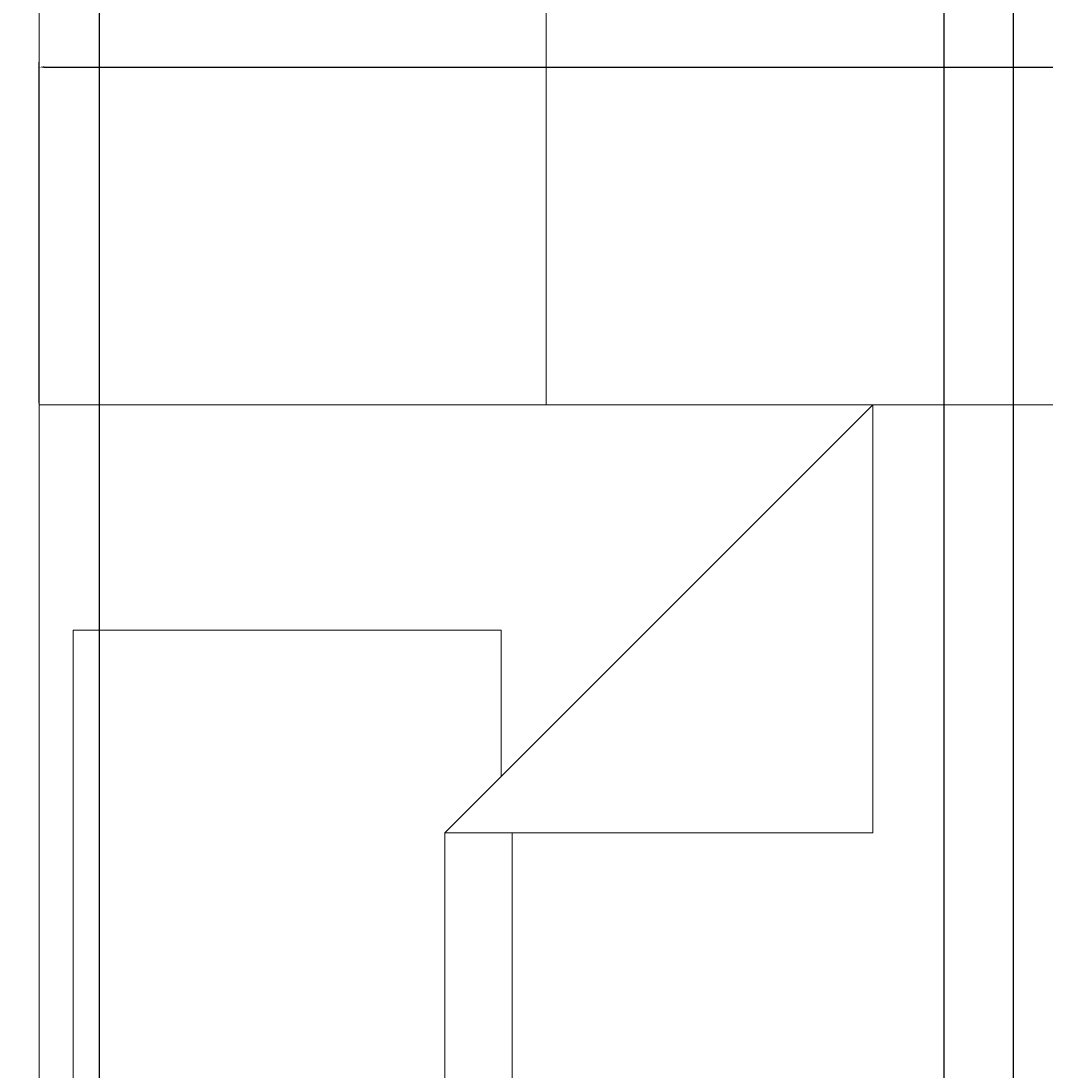
# Model space of a CAD drawing. Units: inches. Extents: x 2231 to 2461, y 2045 to 2455.
# Tile 72 of 95: x 2260 to 2296, y 2372 to 2409. Entities that reach past the tile are written whole.
import ezdxf

# ---------------------------------------------------------------- set-up
doc = ezdxf.new("R2010")
doc.units = ezdxf.units.IN
doc.layers.add('A-ANNO-DIMS', color=2, linetype='Continuous', lineweight=18)
doc.layers.add('A-FURN', color=9, linetype='Continuous', lineweight=18)
doc.styles.get("Standard").update_dxf_attribs({"font": 'arial.ttf'})
doc.dimstyles.get("Standard").update_dxf_attribs({"dimtxt": 0.18, "dimasz": 0.18, "dimexe": 0.18, "dimexo": 0.0625, "dimgap": 0.09, "dimtad": 0, "dimtih": 1, "dimtoh": 1, "dimdec": 4, "dimzin": 0, "dimdsep": 46, "dimtxsty": 'Standard', "dimcen": 0.09, "dimadec": 0, "dimazin": 0, "dimtfac": 1, "dimtdec": 4, "dimtofl": 0, "dimtmove": 0, "dimatfit": 3, "dimfxl": 1, "dimtolj": 1, "dimtzin": 0, "dimarcsym": 0})

# ---------------------------------------------------------------- blocks, each defined once
blk = doc.blocks.new('Bed - Queen')
for p, q in [((0, 0), (59.99999, 0)), ((59.99999, 0), (59.99999, -80.00003)), ((31.19999, -1.2), (51.99999, -1.2)), ((51.99999, -1.2), (51.99999, -16.4)), ((0, -14.4), (44.8, -14.4)), ((59.99999, -29.6), (44.8, -14.4)), ((44.8, -14.4), (44.8, -29.6)), ((51.99999, -16.4), (46.79936, -16.4)), ((44.8, -16.8), (0, -16.8)), ((44.8, -29.6), (59.99999, -29.6))]:
    blk.add_line(p, q)
blk = doc.blocks.new('NIGHTSTAND-18IN')
blk.add_lwpolyline([(0, 0), (18, 0), (18, 18), (0, 18)], close=True)
blk = doc.blocks.new('*D19')
at = {"layer": 'A-ANNO-DIMS', "color": 0, "lineweight": -2, "transparency": 16777216}
for p, q in [((2260.188, 2395.316), (2260.188, 2407.433)), ((2260.368, 2407.253), (2299.194, 2407.253)), ((2340.008, 2407.253), (2301.182, 2407.253)), ((2340.188, 2395.316), (2340.188, 2407.433))]:
    blk.add_line(p, q, dxfattribs=at)
at = {"layer": 'A-ANNO-DIMS', "color": 0, "transparency": 16777216}
for points in [[(2260.368, 2407.283), (2260.368, 2407.223), (2260.188, 2407.253)], [(2340.008, 2407.283), (2340.008, 2407.223), (2340.188, 2407.253)]]:
    blk.add_solid(points, dxfattribs=at)
at = {"layer": 'Defpoints', "color": 0, "transparency": 16777216}
for p in [(2260.188, 2407.253), (2260.188, 2395.253), (2340.188, 2395.253)]:
    blk.add_point(p, dxfattribs=at)
at = {"layer": 'A-ANNO-DIMS', "color": 0, "transparency": 16777216, "insert": (2300.188, 2407.253), "char_height": 0.18, "attachment_point": 5}
blk.add_mtext('\\A1;QUEEN BED 80', dxfattribs=at)
blk = doc.blocks.new('*D47')
at = {"layer": 'A-ANNO-DIMS', "color": 0, "lineweight": -2, "transparency": 16777216}
for p, q in [((2258.794, 2182.895), (2258.794, 2454.645)), ((2294.794, 2182.895), (2294.794, 2454.645)), ((2258.974, 2454.465), (2276.575, 2454.465)), ((2294.614, 2454.465), (2277.012, 2454.465))]:
    blk.add_line(p, q, dxfattribs=at)
at = {"layer": 'A-ANNO-DIMS', "color": 0, "transparency": 16777216}
for points in [[(2258.974, 2454.495), (2258.974, 2454.435), (2258.794, 2454.465)], [(2294.614, 2454.495), (2294.614, 2454.435), (2294.794, 2454.465)]]:
    blk.add_solid(points, dxfattribs=at)
at = {"layer": 'Defpoints', "color": 0, "transparency": 16777216}
for p in [(2294.794, 2454.465), (2258.794, 2182.833), (2294.794, 2182.833)]:
    blk.add_point(p, dxfattribs=at)
at = {"layer": 'A-ANNO-DIMS', "color": 0, "transparency": 16777216, "insert": (2276.794, 2454.465), "char_height": 0.18, "attachment_point": 5}
blk.add_mtext('\\A1;36', dxfattribs=at)
blk = doc.blocks.new('*D62')
at = {"layer": 'A-ANNO-DIMS', "color": 0, "lineweight": -2, "transparency": 16777216}
for p, q in [((2262.321, 2255.176), (2262.321, 2454.645)), ((2292.321, 2253.176), (2292.321, 2454.645)), ((2262.501, 2454.465), (2277.102, 2454.465)), ((2292.141, 2454.465), (2277.539, 2454.465))]:
    blk.add_line(p, q, dxfattribs=at)
at = {"layer": 'A-ANNO-DIMS', "color": 0, "transparency": 16777216}
for points in [[(2262.501, 2454.495), (2262.501, 2454.435), (2262.321, 2454.465)], [(2292.141, 2454.495), (2292.141, 2454.435), (2292.321, 2454.465)]]:
    blk.add_solid(points, dxfattribs=at)
at = {"layer": 'Defpoints', "color": 0, "transparency": 16777216}
for p in [(2292.321, 2454.465), (2262.321, 2255.114), (2292.321, 2253.114)]:
    blk.add_point(p, dxfattribs=at)
at = {"layer": 'A-ANNO-DIMS', "color": 0, "transparency": 16777216, "insert": (2277.321, 2454.465), "char_height": 0.18, "attachment_point": 5}
blk.add_mtext('\\A1;30', dxfattribs=at)

msp = doc.modelspace()

# ---------------------------------------------------------------- block references
at = {"layer": 'A-FURN'}
msp.add_blockref('NIGHTSTAND-18IN', (2260.188, 2395.253), dxfattribs=at)
at = {"layer": 'A-FURN', "rotation": 90}
msp.add_blockref('Bed - Queen', (2260.1881, 2335.2534), dxfattribs=at)

# ---------------------------------------------------------------- dimensions: what is measured, and where the dimension line sits
at = {"layer": 'A-ANNO-DIMS'}
for base, p1, p2, picture, middle in [((2294.7935, 2454.4653), (2258.7935, 2182.8328), (2294.7935, 2182.8328), '*D47', (2276.7935, 2454.4653)), ((2292.3207, 2454.4653), (2262.3207, 2255.1137), (2292.3207, 2253.1137), '*D62', (2277.3207, 2454.4653))]:
    dim = msp.add_linear_dim(base=base, p1=p1, p2=p2, dimstyle='Standard', override={"dimdec": 0, "dimlfac": 1, "dimrnd": 0, "dimzin": 0, "dimdsep": 46, "dimlunit": 2}, dxfattribs=at)
    dim.commit()
    dim.dimension.update_dxf_attribs({"geometry": picture, "text_midpoint": middle})
dim = msp.add_linear_dim(base=(2260.1881, 2407.2534), p1=(2340.1882, 2395.2534), p2=(2260.1881, 2395.2534), angle=180, text='QUEEN BED <>', dimstyle='Standard', override={"dimdec": 0, "dimlfac": 1, "dimrnd": 0, "dimzin": 0, "dimdsep": 46, "dimlunit": 2}, dxfattribs=at)
dim.commit()
dim.dimension.update_dxf_attribs({"geometry": '*D19', "text_midpoint": (2300.1882, 2407.2534)})

doc.saveas('drawing.dxf')
